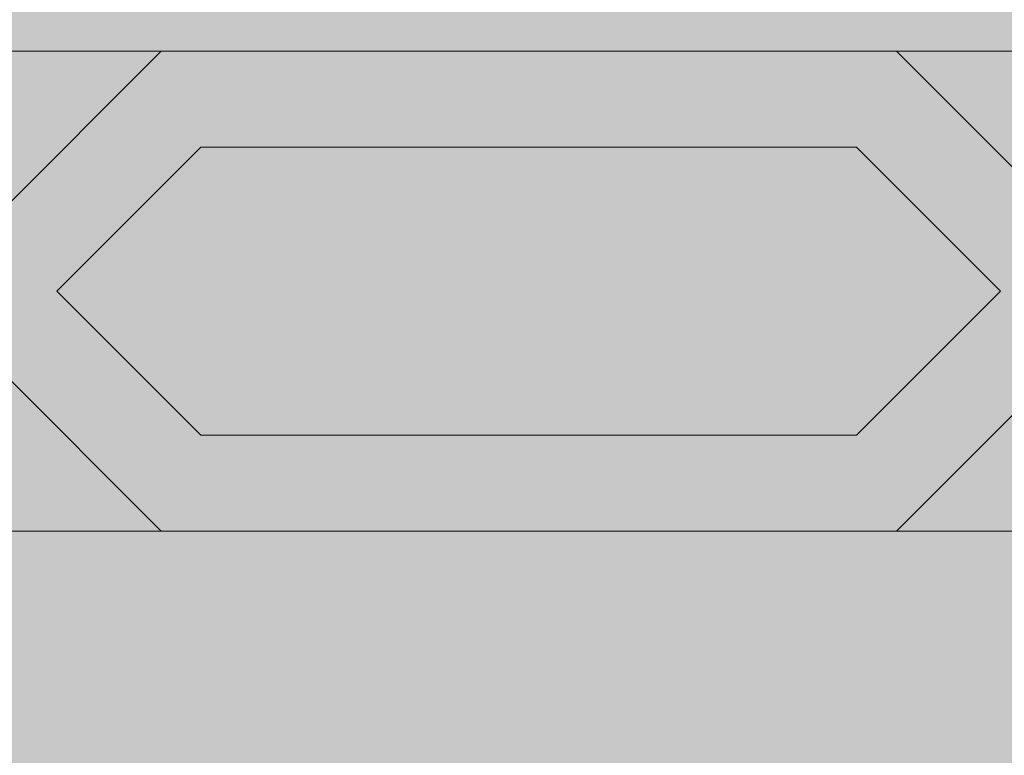
# Model space of a CAD drawing. Units: inches. Extents: x 844 to 2234, y 346 to 1084.
# Tile 81 of 93: x 2003.94 to 2006.557, y 710.971 to 712.926. Entities that reach past the tile are written whole.
import ezdxf

# ---------------------------------------------------------------- set-up
doc = ezdxf.new("R2010")
doc.units = ezdxf.units.IN
doc.header["$MEASUREMENT"] = 0
for name, color, linetype, lineweight in [('A-ANNO-DIMS', 2, 'Continuous', 18), ('furniture', 8, 'Continuous', 18), ('RA-AP-01$0$INT', 35, 'Continuous', 5)]:
    doc.layers.add(name, color=color, linetype=linetype, lineweight=lineweight)
doc.layers.add('RA-AP-01$0$FURN', color=3, linetype='Continuous')
doc.styles.get("Standard").update_dxf_attribs({"font": 'arial.ttf'})
doc.dimstyles.get("Standard").update_dxf_attribs({"dimtxt": 6, "dimasz": 3, "dimexe": 0.18, "dimexo": 0.0625, "dimgap": 0.09, "dimtad": 0, "dimtih": 1, "dimtoh": 1, "dimdec": 1, "dimzin": 0, "dimdsep": 46, "dimlunit": 3, "dimtxsty": 'Standard', "dimblk": 'ARCHTICK', "dimcen": 0.09, "dimadec": 0, "dimazin": 0, "dimtfac": 1, "dimtdec": 1, "dimtofl": 0, "dimtmove": 0, "dimatfit": 3, "dimfxl": 1, "dimtolj": 1, "dimtzin": 0, "dimarcsym": 0})

# ---------------------------------------------------------------- blocks, each defined once
blk = doc.blocks.new('A$C18D01794')
at = {"layer": 'RA-AP-01$0$INT'}
h = blk.add_hatch(color=256, dxfattribs=at)
h.paths.add_polyline_path([(4.355206456958071, -6.156712009588037), (4.355206456958071, -8.056712009588038), (5.455206456958072, -8.056712009588038), (5.455206456958072, -6.156712009588037)])
h.paths.add_polyline_path([(4.405206456958072, -8.006712009588039), (4.405206456958072, -6.206712009588038), (5.405206456958072, -6.206712009588038), (5.405206456958072, -8.006712009588039)], flags=16)
h = blk.add_hatch(color=256, dxfattribs=at)
h.paths.add_polyline_path([(4.505206456958071, -7.585498806127123), (4.46934859260189, -7.549640941759413), (4.505206456958071, -7.513783077414768), (4.505206456958071, -7.381963272220687), (4.469348592616735, -7.346105407867824), (4.505206456958071, -7.310247543514964), (4.505206456958071, -7.178427738324996), (4.469348592586679, -7.142569873965138), (4.505206456952245, -7.106712009588038), (4.476922185709333, -7.106712009588038), (4.455206456960671, -7.128427738343681), (4.433490728198047, -7.106712009588038), (4.405206456946033, -7.106712009588036), (4.441064321339216, -7.142569873969684), (4.40520645695807, -7.178427738362358), (4.405206456958072, -7.310247543472698), (4.441064321364728, -7.346105407867826), (4.40520645695807, -7.381963272262947), (4.40520645695807, -7.513783077378263), (4.441064321354429, -7.549640941786153), (4.405206456958072, -7.585498806170974), (4.405206456958072, -7.717318611286652), (4.441064321333084, -7.753176475673194), (4.405206456958072, -7.789034340036673), (4.405206456958072, -8.006712009588039), (4.644348592588106, -8.006712009588039), (4.680206456964639, -7.970854145211967), (4.716064321341165, -8.006712009588039), (4.869348592586113, -8.006712009588039), (4.905206456964143, -7.970854145210465), (4.941064321342174, -8.006712009588039), (5.094348592587118, -8.006712009588037), (5.130206456963649, -7.970854145211967), (5.166064321340178, -8.006712009588039), (5.405206456958072, -8.006712009588039), (5.405206456958072, -7.789034340024526), (5.369348592595202, -7.753176475673196), (5.40520645695807, -7.717318611298797), (5.40520645695807, -7.585498806158829), (5.369348592573859, -7.549640941786151), (5.40520645695807, -7.51378307739041), (5.40520645695807, -7.381963272250803), (5.36934859256356, -7.346105407867824), (5.405206456958072, -7.310247543484846), (5.405206456958072, -7.178427738350217), (5.369348592589068, -7.142569873969682), (5.405206456982249, -7.106712009588038), (5.376922185730244, -7.106712009588038), (5.355206456967613, -7.128427738343679), (5.333490728218955, -7.10671200958804), (5.305206456976043, -7.106712009588042), (5.341064321341609, -7.142569873965136), (5.305206456958072, -7.178427738337141), (5.305206456958072, -7.310247543502816), (5.34106432131155, -7.346105407867824), (5.305206456958072, -7.381963272232832), (5.30520645695807, -7.513783077402624), (5.341064321326395, -7.549640941759413), (5.305206456958072, -7.585498806139263), (5.305206456958072, -7.717318611299605), (5.341064321347738, -7.753176475677737), (5.305206456958072, -7.78903434007894), (5.30520645695807, -7.906712009588039), (5.166064321336834, -7.906712009588039), (5.130206456963647, -7.942569873961684), (5.094348592590464, -7.906712009588039), (4.941064321338827, -7.906712009588041), (4.905206456964145, -7.942569873963183), (4.869348592589459, -7.906712009588039), (4.716064321337822, -7.906712009588041), (4.680206456964641, -7.942569873961684), (4.644348592591453, -7.906712009588039), (4.505206456958071, -7.906712009588039), (4.505206456958071, -7.789034340066795), (4.469348592580545, -7.753176475677738), (4.505206456958071, -7.717318611311748)])
h.paths.add_polyline_path([(4.485206456974132, -7.709034340046354), (4.45520645695909, -7.739034340051736), (4.425206456974128, -7.709034340057131), (4.425206456993394, -7.593783077384998), (4.45520645699153, -7.563783077396511), (4.485206456993396, -7.593783077408017)], flags=16)
h.paths.add_polyline_path([(4.455206456954537, -7.767318611299197), (4.485206456958242, -7.797318611312542), (4.48520645695951, -7.912569873958716), (4.45520645695415, -7.942569873954422), (4.425206456957888, -7.912569873967813), (4.425206456957888, -7.797318611286197)], flags=16)
h.paths.add_polyline_path([(4.455206456964794, -7.535498806149051), (4.42520645696469, -7.5054988061393), (4.425206456983954, -7.390247543486406), (4.455206456990734, -7.360247543489279), (4.485206456983953, -7.39024754349214), (4.485206456964687, -7.505498806158811)], flags=16)
h.paths.add_polyline_path([(4.499348592588947, -7.926712009585049), (4.636064321340932, -7.926712009585049), (4.666064321342317, -7.956712009586821), (4.636064321343707, -7.986712009585048), (4.499348592575121, -7.986712009585048), (4.469348592591685, -7.956712009591957)], flags=16)
h.paths.add_polyline_path([(4.425206456957888, -7.940854145195974), (4.471064321332215, -7.986712009585049), (4.425206456957888, -7.986712009585049)], flags=16)
h.paths.add_polyline_path([(4.455206456990734, -7.331963272246367), (4.425206456989053, -7.301963272254337), (4.425206456969784, -7.186712009596224), (4.455206456965226, -7.156712009591144), (4.485206456969787, -7.186712009586051), (4.485206456989053, -7.301963272238404)], flags=16)
h.paths.add_polyline_path([(4.72434859258714, -7.926712009586255), (4.861064321340141, -7.926712009586248), (4.891064321340324, -7.956712009586823), (4.861064321340513, -7.986712009586252), (4.724348592586768, -7.986712009586252), (4.694348592586956, -7.956712009586821)], flags=16)
h.paths.add_polyline_path([(4.919348592587961, -7.956712009586821), (4.949348592588145, -7.92671200958625), (5.08606432134115, -7.926712009586253), (5.116064321341327, -7.956712009586823), (5.086064321341519, -7.986712009586252), (4.949348592587774, -7.986712009586252)], flags=16)
h.paths.add_polyline_path([(5.144348592585967, -7.956712009586823), (5.174348592587358, -7.926712009585049), (5.311064321339338, -7.926712009585049), (5.3410643213366, -7.956712009591957), (5.311064321353163, -7.986712009585048), (5.174348592584576, -7.986712009585048)], flags=16)
h.paths.add_polyline_path([(5.32520645693489, -7.593783077408021), (5.355206456936755, -7.563783077396511), (5.385206456934894, -7.593783077384998), (5.38520645695416, -7.709034340057128), (5.355206456969194, -7.739034340051736), (5.325206456954153, -7.709034340046352)], flags=16)
h.paths.add_polyline_path([(5.325206456970042, -7.797318611312542), (5.355206456973747, -7.767318611299197), (5.385206456970398, -7.7973186112862), (5.385206456970398, -7.912569873967816), (5.355206456974136, -7.942569873954422), (5.325206456968778, -7.912569873958716)], flags=16)
h.paths.add_polyline_path([(5.325206456963599, -7.505498806158811), (5.325206456944333, -7.39024754349214), (5.355206456937552, -7.360247543489279), (5.385206456944332, -7.39024754348641), (5.385206456963596, -7.505498806139303), (5.355206456963492, -7.53549880614905)], flags=16)
h.paths.add_polyline_path([(5.32520645693923, -7.301963272238403), (5.3252064569585, -7.186712009586051), (5.355206456963062, -7.156712009591142), (5.3852064569585, -7.186712009596224), (5.385206456939234, -7.301963272254338), (5.355206456937552, -7.331963272246369)], flags=16)
h.paths.add_polyline_path([(5.339348592596071, -7.986712009585048), (5.385206456970398, -7.940854145195972), (5.385206456970396, -7.986712009585048)], flags=16)
h = blk.add_hatch(color=256, dxfattribs=at)
h.paths.add_polyline_path([(4.469348592586677, -7.142569873965136), (4.505206456958073, -7.178427738324996), (4.505206456958071, -7.106712009582215)])
h.paths.add_polyline_path([(4.455206456960671, -7.128427738343681), (4.476922185709333, -7.106712009588038), (4.433490728198045, -7.106712009588038)])
h.paths.add_polyline_path([(4.405206456958073, -7.178427738362358), (4.441064321339218, -7.142569873969684), (4.40520645695807, -7.106712009600073)])
h.paths.add_polyline_path([(4.425206456989053, -7.301963272254335), (4.455206456990736, -7.331963272246371), (4.485206456989055, -7.301963272238399), (4.48520645696979, -7.186712009586054), (4.455206456965227, -7.15671200959114), (4.425206456969784, -7.186712009596224)])
h.paths.add_polyline_path([(4.505206456958073, -7.381963272220689), (4.505206456958071, -7.310247543514961), (4.469348592616738, -7.346105407867826)])
h.paths.add_polyline_path([(4.425206456964688, -7.5054988061393), (4.455206456964794, -7.535498806149051), (4.485206456964689, -7.505498806158811), (4.485206456983951, -7.390247543492138), (4.455206456990736, -7.360247543489277), (4.425206456983956, -7.39024754348641)])
h.paths.add_polyline_path([(4.425206456974126, -7.709034340057128), (4.455206456959092, -7.739034340051736), (4.485206456974132, -7.709034340046356), (4.485206456993396, -7.593783077408017), (4.45520645699153, -7.563783077396511), (4.425206456993394, -7.593783077384999)])
h.paths.add_polyline_path([(4.46934859260189, -7.549640941759415), (4.505206456958071, -7.585498806127123), (4.505206456958073, -7.513783077414766)])
h.paths.add_polyline_path([(4.405206456958073, -7.585498806170972), (4.441064321354427, -7.549640941786151), (4.405206456958072, -7.513783077378263)])
h.paths.add_polyline_path([(4.405206456958072, -7.789034340036673), (4.441064321333084, -7.753176475673194), (4.405206456958072, -7.71731861128665)])
h.paths.add_polyline_path([(4.469348592580547, -7.75317647567774), (4.505206456958071, -7.789034340066795), (4.505206456958071, -7.717318611311744)])
h.paths.add_polyline_path([(4.425206456957888, -7.912569873967814), (4.45520645695415, -7.942569873954422), (4.485206456959507, -7.912569873958718), (4.48520645695824, -7.797318611312542), (4.455206456954537, -7.767318611299197), (4.425206456957888, -7.797318611286202)])
h.paths.add_polyline_path([(4.425206456957888, -7.986712009585049), (4.471064321332215, -7.986712009585049), (4.425206456957888, -7.940854145195972)])
h.paths.add_polyline_path([(4.499348592575121, -7.986712009585048), (4.636064321343707, -7.986712009585049), (4.666064321342317, -7.956712009586823), (4.636064321340932, -7.926712009585049), (4.499348592588945, -7.926712009585049), (4.469348592591685, -7.95671200959196)])
h.paths.add_polyline_path([(4.680206456964641, -7.942569873961684), (4.716064321337824, -7.906712009588039), (4.644348592591454, -7.906712009588039)])
h.paths.add_polyline_path([(4.644348592588108, -8.006712009588039), (4.716064321341167, -8.006712009588039), (4.680206456964637, -7.970854145211964)])
h.paths.add_polyline_path([(4.724348592586768, -7.98671200958625), (4.861064321340514, -7.986712009586252), (4.891064321340324, -7.956712009586819), (4.861064321340141, -7.92671200958625), (4.724348592587134, -7.926712009586255), (4.694348592586957, -7.956712009586821)])
h.paths.add_polyline_path([(4.905206456964143, -7.942569873963183), (4.941064321338827, -7.906712009588039), (4.869348592589457, -7.906712009588037)])
h.paths.add_polyline_path([(4.869348592586113, -8.006712009588039), (4.941064321342172, -8.006712009588037), (4.905206456964145, -7.970854145210463)])
h.paths.add_polyline_path([(4.949348592587774, -7.986712009586252), (5.086064321341521, -7.986712009586252), (5.116064321341329, -7.956712009586823), (5.08606432134115, -7.926712009586253), (4.949348592588145, -7.92671200958625), (4.919348592587961, -7.956712009586819)])
h.paths.add_polyline_path([(5.130206456963645, -7.942569873961684), (5.166064321336834, -7.906712009588039), (5.094348592590464, -7.906712009588039)])
h.paths.add_polyline_path([(5.094348592587119, -8.006712009588039), (5.166064321340178, -8.006712009588039), (5.130206456963651, -7.970854145211967)])
h.paths.add_polyline_path([(5.174348592584578, -7.986712009585048), (5.311064321353163, -7.986712009585048), (5.341064321336602, -7.956712009591958), (5.31106432133934, -7.926712009585049), (5.174348592587352, -7.926712009585049), (5.144348592585969, -7.956712009586823)])
h.paths.add_polyline_path([(5.325206456968778, -7.912569873958718), (5.355206456974136, -7.942569873954422), (5.385206456970396, -7.912569873967814), (5.385206456970396, -7.797318611286199), (5.355206456973747, -7.767318611299197), (5.325206456970044, -7.797318611312544)])
h.paths.add_polyline_path([(5.339348592596073, -7.986712009585048), (5.385206456970396, -7.986712009585049), (5.385206456970398, -7.94085414519597)])
h.paths.add_polyline_path([(5.325206456954155, -7.709034340046354), (5.355206456969194, -7.739034340051734), (5.38520645695416, -7.709034340057128), (5.385206456934896, -7.593783077384999), (5.355206456936758, -7.563783077396513), (5.325206456934888, -7.593783077408019)])
h.paths.add_polyline_path([(5.305206456958072, -7.789034340078938), (5.341064321347739, -7.753176475677738), (5.305206456958072, -7.717318611299605)])
h.paths.add_polyline_path([(5.369348592595204, -7.753176475673194), (5.40520645695807, -7.789034340024526), (5.405206456958072, -7.717318611298798)])
h.paths.add_polyline_path([(5.405206456958072, -7.585498806158831), (5.405206456958072, -7.513783077390407), (5.369348592573857, -7.549640941786151)])
h.paths.add_polyline_path([(5.305206456958072, -7.585498806139266), (5.341064321326393, -7.549640941759413), (5.305206456958072, -7.513783077402626)])
h.paths.add_polyline_path([(5.325206456963599, -7.50549880615881), (5.355206456963494, -7.535498806149055), (5.385206456963598, -7.505498806139302), (5.385206456944334, -7.390247543486411), (5.355206456937552, -7.360247543489279), (5.325206456944333, -7.39024754349214)])
h.paths.add_polyline_path([(5.305206456958072, -7.38196327223283), (5.341064321311551, -7.346105407867824), (5.305206456958072, -7.31024754350282)])
h.paths.add_polyline_path([(5.325206456939231, -7.301963272238404), (5.355206456937552, -7.331963272246369), (5.385206456939235, -7.301963272254335), (5.385206456958502, -7.186712009596224), (5.355206456963061, -7.156712009591142), (5.3252064569585, -7.186712009586051)])
h.paths.add_polyline_path([(5.404581768715993, -7.381338584008926, -0.001217816984214), (5.405206456958072, -7.381112009582329), (5.405206456958072, -7.310247543484846), (5.369348592563558, -7.346105407867826)])
h.paths.add_polyline_path([(5.36934859258907, -7.142569873969684), (5.40520645695807, -7.178427738350215), (5.405206456958072, -7.106712009612218)])
h.paths.add_polyline_path([(5.355206456967613, -7.128427738343683), (5.376922185730239, -7.106712009588038), (5.333490728218953, -7.10671200958804)])
h.paths.add_polyline_path([(5.30520645695807, -7.178427738337139), (5.341064321341609, -7.142569873965134), (5.305206456958074, -7.10671200957007)])
blk.add_hatch(color=256, dxfattribs=at).paths.add_polyline_path([(4.505206456958071, -7.906712009588039), (5.305206456958072, -7.906712009588039), (5.305206456958072, -7.106712009588038), (5.255206456951893, -7.106712009588036), (5.25520645694868, -7.856712009570104), (4.555206456959269, -7.856712009588616), (4.555206456956052, -7.106712009588038), (4.505206456958073, -7.106712009588038)])
for p, q in [((5.267206456961765, -7.906712009586254), (4.543206456966523, -7.906712009586254)), ((5.2672064569642, -7.906712009586255), (4.54320645696085, -7.906712009586255)), ((4.716064321339607, -7.906712009586254), (4.680206456964639, -7.942569873961684)), ((4.869348592587674, -7.906712009586254), (4.905206456964143, -7.942569873963183)), ((4.724348592587136, -7.926712009586253), (4.694348592586957, -7.956712009586823)), ((4.861064321340141, -7.92671200958625), (4.724348592587136, -7.926712009586253)), ((4.861064321340141, -7.92671200958625), (4.891064321340324, -7.956712009586821)), ((4.724348592586768, -7.986712009586252), (4.694348592586957, -7.956712009586823)), ((4.861064321340513, -7.986712009586252), (4.891064321340324, -7.956712009586821)), ((4.716064321339382, -8.006712009586252), (4.680206456964637, -7.970854145211966)), ((4.8693485925879, -8.006712009586252), (4.905206456964143, -7.970854145210465)), ((4.861064321340513, -7.986712009586252), (4.724348592586768, -7.986712009586252))]:
    blk.add_line(p, q, dxfattribs=at)
for points in [[(5.405206456958072, -8.006712009588039), (4.405206456958072, -8.006712009588039), (4.405206456958072, -7.106712009588038)], [(5.305206456958072, -7.106712009588038), (5.305206456958072, -7.906712009588039), (4.505206456958071, -7.906712009588039), (4.505206456958071, -7.106712009588038)]]:
    blk.add_lwpolyline(points, dxfattribs=at)
blk = doc.blocks.new('A$C5D2F253E')
at = {"layer": 'RA-AP-01$0$FURN', "xscale": -0.7999999999883585, "yscale": 0.7999999999883585, "zscale": 0.8, "rotation": 90}
blk.add_blockref('A$C18D01794', (-5.687757199772477, 4.75791982714071), dxfattribs=at)
blk = doc.blocks.new('_ArchTick')
at = {"color": 0, "linetype": 'ByBlock', "const_width": 0.15}
blk.add_lwpolyline([(-0.5, -0.5), (0.5, 0.5)], dxfattribs=at)
blk = doc.blocks.new('*D121')
at = {"layer": 'A-ANNO-DIMS', "color": 0, "lineweight": -2, "transparency": 16777216}
for p, q in [((2030.271987351997, 734.262611118704), (2040.245275089302, 734.262611118704)), ((2040.065275089302, 734.262611118704), (2040.065275089302, 704.6043509484256)), ((2040.065275089302, 668.557359536674), (2040.065275089302, 698.2156197069523)), ((2030.271987351997, 668.557359536674), (2040.245275089302, 668.557359536674))]:
    blk.add_line(p, q, dxfattribs=at)
at = {"layer": 'Defpoints', "color": 0, "transparency": 16777216}
for p in [(2030.209487351997, 734.262611118704), (2040.065275089302, 734.262611118704), (2030.209487351997, 668.557359536674)]:
    blk.add_point(p, dxfattribs=at)
at = {"layer": 'A-ANNO-DIMS', "color": 0, "lineweight": -2, "transparency": 16777216, "xscale": 3, "yscale": 3, "zscale": 3}
for p, rotation in [((2040.065275089302, 734.262611118704), 90), ((2040.065275089302, 668.557359536674), 270)]:
    blk.add_blockref('_ArchTick', p, dxfattribs=dict(at, rotation=rotation))
at = {"layer": 'A-ANNO-DIMS', "color": 0, "transparency": 16777216, "insert": (2040.065275089302, 701.4099853276883), "char_height": 6, "attachment_point": 5}
blk.add_mtext('\\A1;LOUNGE SET 5\'-5 1/2" TYP.', dxfattribs=at)

msp = doc.modelspace()

# ---------------------------------------------------------------- block references
at = {"layer": 'furniture', "xscale": -15.94108302203742, "yscale": 15.94108302203742, "zscale": 15.94108302203742, "rotation": 270}
msp.add_blockref('A$C5D2F253E', (1990.567271852805, 701.4028671565849), dxfattribs=at)

# ---------------------------------------------------------------- dimensions: what is measured, and where the dimension line sits
at = {"layer": 'A-ANNO-DIMS'}
dim = msp.add_linear_dim(base=(2040.065275089302, 734.262611118704), p1=(2030.209487351996, 668.5573595366737), p2=(2030.209487351996, 734.2626111187037), angle=90, text='LOUNGE SET <> TYP.', dimstyle='Standard', override={"dimdec": 1, "dimlfac": 1, "dimrnd": 0, "dimzin": 1, "dimdsep": 46, "dimlunit": 4, "dimfrac": 2}, dxfattribs=at)
dim.commit()
dim.dimension.update_dxf_attribs({"geometry": '*D121', "text_midpoint": (2040.065275089302, 701.4099853276883)})

doc.saveas('drawing.dxf')
